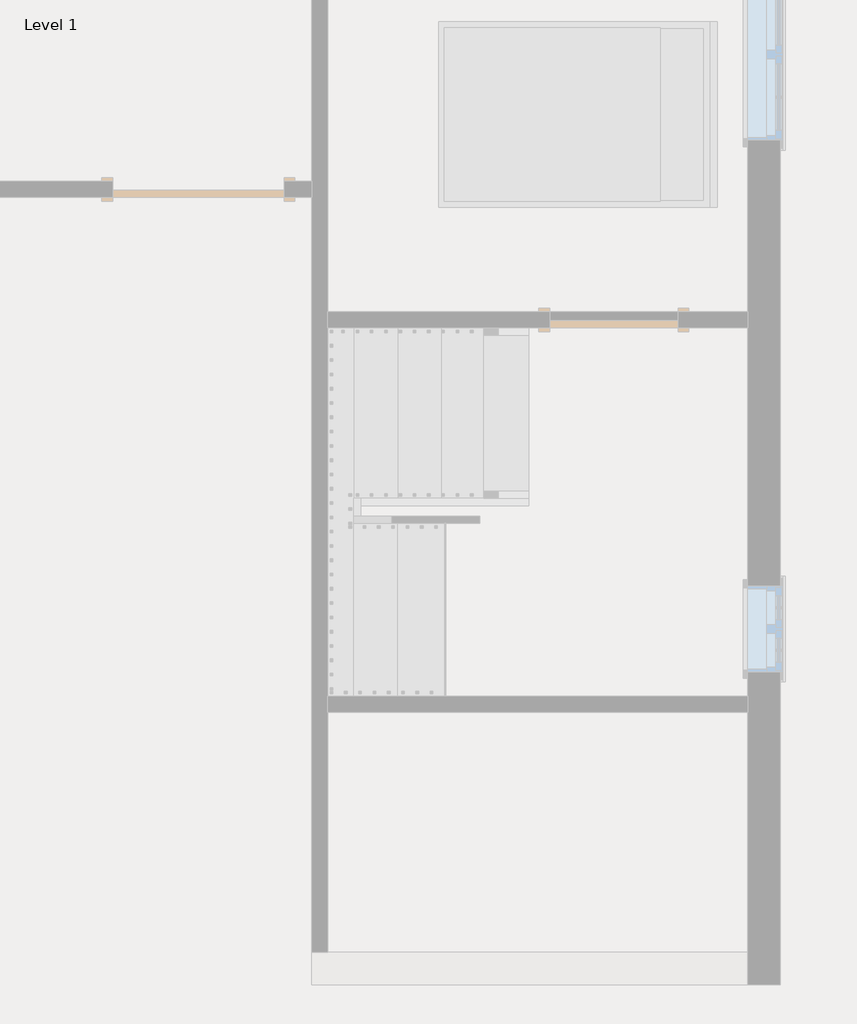
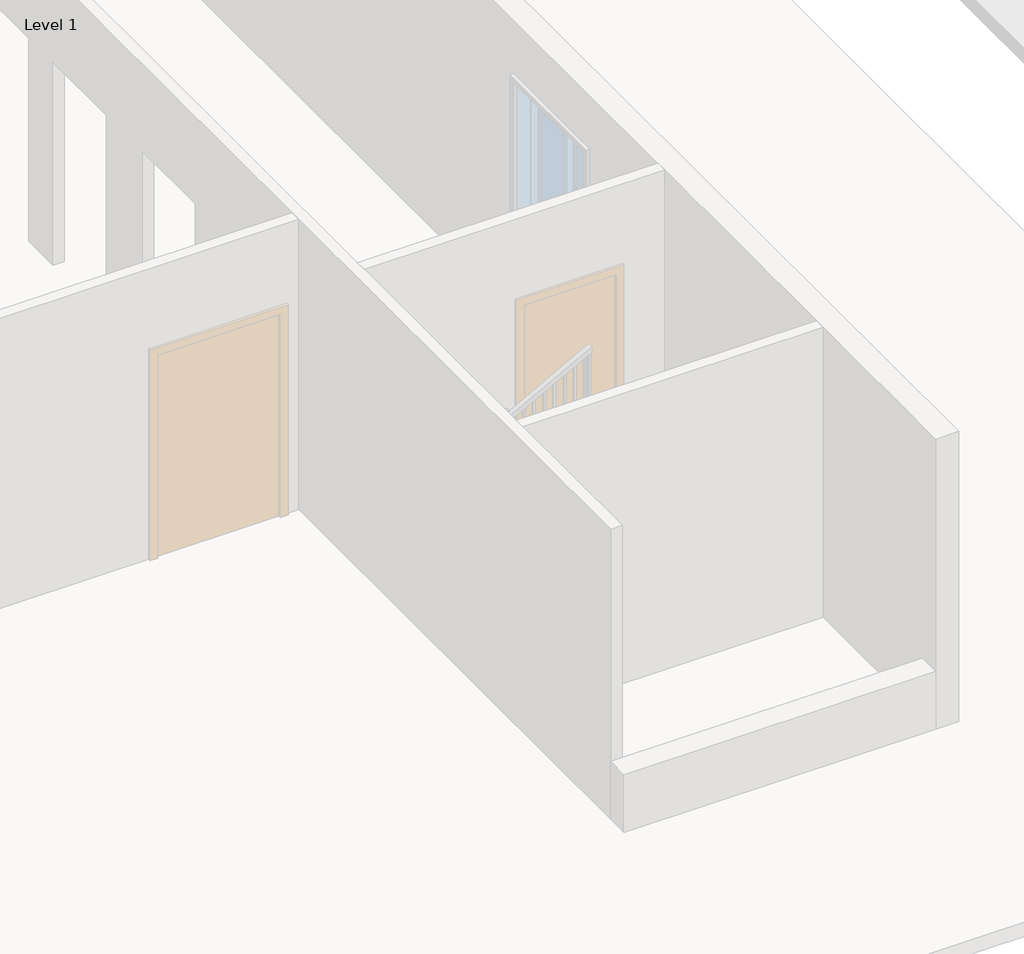
# One storey, part 5 of 7: 2 railings.
"""IFC4 building model written with IfcOpenShell, lengths in millimetres."""

from ifc_helpers import new_model, si_unit, frame, origin, place, context, project, spatial, polyline, outline, extrude, faceted_brep, element, save

model = new_model("IFC4")

# Units and contexts
model_context = context("Model", 3, world=origin())
ifc_project = project(units=[si_unit("LENGTHUNIT", "METRE", prefix="MILLI")], contexts=[model_context])

# Site, building, storey
site = spatial("IfcSite", under=ifc_project)
building = spatial("IfcBuilding", under=site)
storey = spatial("IfcBuildingStorey", under=building, Name="Level 1", Elevation=0.0)

# Railings
placement = place(None, origin())
element("IfcRailing", 1, ObjectType="Handrail - Rectangular", at=placement, inside=storey, context=model_context, shape_type="SolidModel", body=[
    faceted_brep([(7105.1820958, 5435.6, 1083.7333333), (7105.1820958, 5435.6, 1025.8977421), (7105.1820958, 5486.4, 1025.8977421), (7105.1820958, 5486.4, 1083.7333333), (5860.5820958, 5435.6, 1761.0666667), (5847.654197, 5435.6, 1710.2666667), (5847.654197, 5486.4, 1710.2666667), (5860.5820958, 5486.4, 1761.0666667), (5727.7, 5435.6, 1761.0666667), (5727.7, 5435.6, 1710.2666667), (5676.9, 5486.4, 1710.2666667), (5676.9, 5486.4, 1761.0666667), (5727.7, 2997.2, 1761.0666667), (5727.7, 2946.4, 1710.2666667), (5676.9, 2946.4, 1710.2666667), (5676.9, 2997.2, 1761.0666667), (5727.7, 2997.2, 1899.5526009), (5727.7, 2946.4, 1848.7526009), (5676.9, 2946.4, 1848.7526009), (5676.9, 2997.2, 1899.5526009), (5727.7, 2921.0, 1899.5526009), (5727.7, 2921.0, 1848.7526009), (5676.9, 2870.2, 1848.7526009), (5676.9, 2870.2, 1899.5526009), (5803.9, 2921.0, 1899.5526009), (5816.8278988, 2921.0, 1848.7526009), (5816.8278988, 2870.2, 1848.7526009), (5803.9, 2870.2, 1899.5526009), (7105.1820958, 2921.0, 2607.7333333), (7105.1820958, 2870.2, 2607.7333333), (7105.1820958, 2870.2, 2549.8977421), (7105.1820958, 2921.0, 2549.8977421)], [[[0, 1, 2, 3]], [[1, 0, 4, 5]], [[2, 1, 5, 6]], [[3, 2, 6, 7]], [[0, 3, 7, 4]], [[5, 4, 8, 9]], [[6, 5, 9, 10]], [[7, 6, 10, 11]], [[4, 7, 11, 8]], [[9, 8, 12, 13]], [[10, 9, 13, 14]], [[11, 10, 14, 15]], [[8, 11, 15, 12]], [[13, 12, 16, 17]], [[14, 13, 17, 18]], [[15, 14, 18, 19]], [[12, 15, 19, 16]], [[17, 16, 20, 21]], [[18, 17, 21, 22]], [[19, 18, 22, 23]], [[16, 19, 23, 20]], [[21, 20, 24, 25]], [[22, 21, 25, 26]], [[23, 22, 26, 27]], [[20, 23, 27, 24]], [[28, 29, 30, 31]], [[25, 24, 28, 31]], [[26, 25, 31, 30]], [[27, 26, 30, 29]], [[24, 27, 29, 28]]]),
    extrude(outline(polyline([(2510.4108873, 7032.625), (2500.0435403, 7013.575), (1524.0, 7013.575), (1524.0, 7032.625), (2510.4108873, 7032.625)])), frame((0.0, 2886.075, 0.0), z_axis=(0.0, 1.0, 0.0), x_axis=(0.0, 0.0, 1.0)), (0.0, 0.0, 1.0), 19.05),
    extrude(outline(polyline([(2455.1183703, 6931.025), (2444.7510233, 6911.975), (1524.0, 6911.975), (1524.0, 6931.025), (2455.1183703, 6931.025)])), frame((0.0, 2886.075, 0.0), z_axis=(0.0, 1.0, 0.0), x_axis=(0.0, 0.0, 1.0)), (0.0, 0.0, 1.0), 19.05),
    extrude(outline(polyline([(2399.8258533, 6829.425), (2389.4585063, 6810.375), (1524.0, 6810.375), (1524.0, 6829.425), (2399.8258533, 6829.425)])), frame((0.0, 2886.075, 0.0), z_axis=(0.0, 1.0, 0.0), x_axis=(0.0, 0.0, 1.0)), (0.0, 0.0, 1.0), 19.05),
    extrude(outline(polyline([(2344.5333363, 6727.825), (2334.1659893, 6708.775), (1354.6666667, 6708.775), (1354.6666667, 6727.825), (2344.5333363, 6727.825)])), frame((0.0, 2886.075, 0.0), z_axis=(0.0, 1.0, 0.0), x_axis=(0.0, 0.0, 1.0)), (0.0, 0.0, 1.0), 19.05),
    extrude(outline(polyline([(2289.2408192, 6626.225), (2278.8734723, 6607.175), (1354.6666667, 6607.175), (1354.6666667, 6626.225), (2289.2408192, 6626.225)])), frame((0.0, 2886.075, 0.0), z_axis=(0.0, 1.0, 0.0), x_axis=(0.0, 0.0, 1.0)), (0.0, 0.0, 1.0), 19.05),
    extrude(outline(polyline([(2233.9483022, 6524.625), (2223.5809553, 6505.575), (1354.6666667, 6505.575), (1354.6666667, 6524.625), (2233.9483022, 6524.625)])), frame((0.0, 2886.075, 0.0), z_axis=(0.0, 1.0, 0.0), x_axis=(0.0, 0.0, 1.0)), (0.0, 0.0, 1.0), 19.05),
    extrude(outline(polyline([(2178.6557852, 6423.025), (2168.2884383, 6403.975), (1185.3333333, 6403.975), (1185.3333333, 6423.025), (2178.6557852, 6423.025)])), frame((0.0, 2886.075, 0.0), z_axis=(0.0, 1.0, 0.0), x_axis=(0.0, 0.0, 1.0)), (0.0, 0.0, 1.0), 19.05),
    extrude(outline(polyline([(2123.3632682, 6321.425), (2112.9959213, 6302.375), (1185.3333333, 6302.375), (1185.3333333, 6321.425), (2123.3632682, 6321.425)])), frame((0.0, 2886.075, 0.0), z_axis=(0.0, 1.0, 0.0), x_axis=(0.0, 0.0, 1.0)), (0.0, 0.0, 1.0), 19.05),
    extrude(outline(polyline([(2068.0707512, 6219.825), (2057.7034043, 6200.775), (1185.3333333, 6200.775), (1185.3333333, 6219.825), (2068.0707512, 6219.825)])), frame((0.0, 2886.075, 0.0), z_axis=(0.0, 1.0, 0.0), x_axis=(0.0, 0.0, 1.0)), (0.0, 0.0, 1.0), 19.05),
    extrude(outline(polyline([(2012.7782342, 6118.225), (2002.4108873, 6099.175), (1016.0, 6099.175), (1016.0, 6118.225), (2012.7782342, 6118.225)])), frame((0.0, 2886.075, 0.0), z_axis=(0.0, 1.0, 0.0), x_axis=(0.0, 0.0, 1.0)), (0.0, 0.0, 1.0), 19.05),
    extrude(outline(polyline([(1957.4857172, 6016.625), (1947.1183703, 5997.575), (1016.0, 5997.575), (1016.0, 6016.625), (1957.4857172, 6016.625)])), frame((0.0, 2886.075, 0.0), z_axis=(0.0, 1.0, 0.0), x_axis=(0.0, 0.0, 1.0)), (0.0, 0.0, 1.0), 19.05),
    extrude(outline(polyline([(1902.1932002, 5915.025), (1891.8258533, 5895.975), (1016.0, 5895.975), (1016.0, 5915.025), (1902.1932002, 5915.025)])), frame((0.0, 2886.075, 0.0), z_axis=(0.0, 1.0, 0.0), x_axis=(0.0, 0.0, 1.0)), (0.0, 0.0, 1.0), 19.05),
    extrude(outline(polyline([(1846.9006832, 5813.425), (1836.5333363, 5794.375), (846.6666667, 5794.375), (846.6666667, 5813.425), (1846.9006832, 5813.425)])), frame((0.0, 2886.075, 0.0), z_axis=(0.0, 1.0, 0.0), x_axis=(0.0, 0.0, 1.0)), (0.0, 0.0, 1.0), 19.05),
    extrude(outline(polyline([(5692.775, 2930.525), (5711.825, 2930.525), (5711.825, 2911.475), (5692.775, 2911.475), (5692.775, 2930.525)])), frame((0.0, 0.0, 846.6666667), z_axis=(0.0, 0.0, 1.0), x_axis=(1.0, 0.0, 0.0)), (0.0, 0.0, 1.0), 1002.0859343),
    extrude(outline(polyline([(5692.775, 3032.125), (5711.825, 3032.125), (5711.825, 3013.075), (5692.775, 3013.075), (5692.775, 3032.125)])), frame((0.0, 0.0, 846.6666667), z_axis=(0.0, 0.0, 1.0), x_axis=(1.0, 0.0, 0.0)), (0.0, 0.0, 1.0), 863.6),
    extrude(outline(polyline([(5692.775, 3133.725), (5711.825, 3133.725), (5711.825, 3114.675), (5692.775, 3114.675), (5692.775, 3133.725)])), frame((0.0, 0.0, 846.6666667), z_axis=(0.0, 0.0, 1.0), x_axis=(1.0, 0.0, 0.0)), (0.0, 0.0, 1.0), 863.6),
    extrude(outline(polyline([(5692.775, 3235.325), (5711.825, 3235.325), (5711.825, 3216.275), (5692.775, 3216.275), (5692.775, 3235.325)])), frame((0.0, 0.0, 846.6666667), z_axis=(0.0, 0.0, 1.0), x_axis=(1.0, 0.0, 0.0)), (0.0, 0.0, 1.0), 863.6),
    extrude(outline(polyline([(5692.775, 3336.925), (5711.825, 3336.925), (5711.825, 3317.875), (5692.775, 3317.875), (5692.775, 3336.925)])), frame((0.0, 0.0, 846.6666667), z_axis=(0.0, 0.0, 1.0), x_axis=(1.0, 0.0, 0.0)), (0.0, 0.0, 1.0), 863.6),
    extrude(outline(polyline([(5692.775, 3438.525), (5711.825, 3438.525), (5711.825, 3419.475), (5692.775, 3419.475), (5692.775, 3438.525)])), frame((0.0, 0.0, 846.6666667), z_axis=(0.0, 0.0, 1.0), x_axis=(1.0, 0.0, 0.0)), (0.0, 0.0, 1.0), 863.6),
    extrude(outline(polyline([(5692.775, 3540.125), (5711.825, 3540.125), (5711.825, 3521.075), (5692.775, 3521.075), (5692.775, 3540.125)])), frame((0.0, 0.0, 846.6666667), z_axis=(0.0, 0.0, 1.0), x_axis=(1.0, 0.0, 0.0)), (0.0, 0.0, 1.0), 863.6),
    extrude(outline(polyline([(5692.775, 3641.725), (5711.825, 3641.725), (5711.825, 3622.675), (5692.775, 3622.675), (5692.775, 3641.725)])), frame((0.0, 0.0, 846.6666667), z_axis=(0.0, 0.0, 1.0), x_axis=(1.0, 0.0, 0.0)), (0.0, 0.0, 1.0), 863.6),
    extrude(outline(polyline([(5692.775, 3743.325), (5711.825, 3743.325), (5711.825, 3724.275), (5692.775, 3724.275), (5692.775, 3743.325)])), frame((0.0, 0.0, 846.6666667), z_axis=(0.0, 0.0, 1.0), x_axis=(1.0, 0.0, 0.0)), (0.0, 0.0, 1.0), 863.6),
    extrude(outline(polyline([(5692.775, 3844.925), (5711.825, 3844.925), (5711.825, 3825.875), (5692.775, 3825.875), (5692.775, 3844.925)])), frame((0.0, 0.0, 846.6666667), z_axis=(0.0, 0.0, 1.0), x_axis=(1.0, 0.0, 0.0)), (0.0, 0.0, 1.0), 863.6),
    extrude(outline(polyline([(5692.775, 3946.525), (5711.825, 3946.525), (5711.825, 3927.475), (5692.775, 3927.475), (5692.775, 3946.525)])), frame((0.0, 0.0, 846.6666667), z_axis=(0.0, 0.0, 1.0), x_axis=(1.0, 0.0, 0.0)), (0.0, 0.0, 1.0), 863.6),
    extrude(outline(polyline([(5692.775, 4048.125), (5711.825, 4048.125), (5711.825, 4029.075), (5692.775, 4029.075), (5692.775, 4048.125)])), frame((0.0, 0.0, 846.6666667), z_axis=(0.0, 0.0, 1.0), x_axis=(1.0, 0.0, 0.0)), (0.0, 0.0, 1.0), 863.6),
    extrude(outline(polyline([(5692.775, 4149.725), (5711.825, 4149.725), (5711.825, 4130.675), (5692.775, 4130.675), (5692.775, 4149.725)])), frame((0.0, 0.0, 846.6666667), z_axis=(0.0, 0.0, 1.0), x_axis=(1.0, 0.0, 0.0)), (0.0, 0.0, 1.0), 863.6),
    extrude(outline(polyline([(5692.775, 4251.325), (5711.825, 4251.325), (5711.825, 4232.275), (5692.775, 4232.275), (5692.775, 4251.325)])), frame((0.0, 0.0, 846.6666667), z_axis=(0.0, 0.0, 1.0), x_axis=(1.0, 0.0, 0.0)), (0.0, 0.0, 1.0), 863.6),
    extrude(outline(polyline([(5692.775, 4352.925), (5711.825, 4352.925), (5711.825, 4333.875), (5692.775, 4333.875), (5692.775, 4352.925)])), frame((0.0, 0.0, 846.6666667), z_axis=(0.0, 0.0, 1.0), x_axis=(1.0, 0.0, 0.0)), (0.0, 0.0, 1.0), 863.6),
    extrude(outline(polyline([(5692.775, 4454.525), (5711.825, 4454.525), (5711.825, 4435.475), (5692.775, 4435.475), (5692.775, 4454.525)])), frame((0.0, 0.0, 846.6666667), z_axis=(0.0, 0.0, 1.0), x_axis=(1.0, 0.0, 0.0)), (0.0, 0.0, 1.0), 863.6),
    extrude(outline(polyline([(5692.775, 4556.125), (5711.825, 4556.125), (5711.825, 4537.075), (5692.775, 4537.075), (5692.775, 4556.125)])), frame((0.0, 0.0, 846.6666667), z_axis=(0.0, 0.0, 1.0), x_axis=(1.0, 0.0, 0.0)), (0.0, 0.0, 1.0), 863.6),
    extrude(outline(polyline([(5692.775, 4657.725), (5711.825, 4657.725), (5711.825, 4638.675), (5692.775, 4638.675), (5692.775, 4657.725)])), frame((0.0, 0.0, 846.6666667), z_axis=(0.0, 0.0, 1.0), x_axis=(1.0, 0.0, 0.0)), (0.0, 0.0, 1.0), 863.6),
    extrude(outline(polyline([(5692.775, 4759.325), (5711.825, 4759.325), (5711.825, 4740.275), (5692.775, 4740.275), (5692.775, 4759.325)])), frame((0.0, 0.0, 846.6666667), z_axis=(0.0, 0.0, 1.0), x_axis=(1.0, 0.0, 0.0)), (0.0, 0.0, 1.0), 863.6),
    extrude(outline(polyline([(5692.775, 4860.925), (5711.825, 4860.925), (5711.825, 4841.875), (5692.775, 4841.875), (5692.775, 4860.925)])), frame((0.0, 0.0, 846.6666667), z_axis=(0.0, 0.0, 1.0), x_axis=(1.0, 0.0, 0.0)), (0.0, 0.0, 1.0), 863.6),
    extrude(outline(polyline([(5692.775, 4962.525), (5711.825, 4962.525), (5711.825, 4943.475), (5692.775, 4943.475), (5692.775, 4962.525)])), frame((0.0, 0.0, 846.6666667), z_axis=(0.0, 0.0, 1.0), x_axis=(1.0, 0.0, 0.0)), (0.0, 0.0, 1.0), 863.6),
    extrude(outline(polyline([(5692.775, 5064.125), (5711.825, 5064.125), (5711.825, 5045.075), (5692.775, 5045.075), (5692.775, 5064.125)])), frame((0.0, 0.0, 846.6666667), z_axis=(0.0, 0.0, 1.0), x_axis=(1.0, 0.0, 0.0)), (0.0, 0.0, 1.0), 863.6),
    extrude(outline(polyline([(5692.775, 5165.725), (5711.825, 5165.725), (5711.825, 5146.675), (5692.775, 5146.675), (5692.775, 5165.725)])), frame((0.0, 0.0, 846.6666667), z_axis=(0.0, 0.0, 1.0), x_axis=(1.0, 0.0, 0.0)), (0.0, 0.0, 1.0), 863.6),
    extrude(outline(polyline([(5692.775, 5267.325), (5711.825, 5267.325), (5711.825, 5248.275), (5692.775, 5248.275), (5692.775, 5267.325)])), frame((0.0, 0.0, 846.6666667), z_axis=(0.0, 0.0, 1.0), x_axis=(1.0, 0.0, 0.0)), (0.0, 0.0, 1.0), 863.6),
    extrude(outline(polyline([(5692.775, 5368.925), (5711.825, 5368.925), (5711.825, 5349.875), (5692.775, 5349.875), (5692.775, 5368.925)])), frame((0.0, 0.0, 846.6666667), z_axis=(0.0, 0.0, 1.0), x_axis=(1.0, 0.0, 0.0)), (0.0, 0.0, 1.0), 863.6),
    extrude(outline(polyline([(5793.9070958, 5470.525), (5793.9070958, 5451.475), (5774.8570958, 5451.475), (5774.8570958, 5470.525), (5793.9070958, 5470.525)])), frame((0.0, 0.0, 846.6666667), z_axis=(0.0, 0.0, 1.0), x_axis=(1.0, 0.0, 0.0)), (0.0, 0.0, 1.0), 863.6),
    extrude(outline(polyline([(1684.2242727, 5895.5070958), (1694.5916197, 5876.4570958), (677.3333333, 5876.4570958), (677.3333333, 5895.5070958), (1684.2242727, 5895.5070958)])), frame((0.0, 5451.475, 0.0), z_axis=(0.0, 1.0, 0.0), x_axis=(0.0, 0.0, 1.0)), (0.0, 0.0, 1.0), 19.05),
    extrude(outline(polyline([(1628.9317557, 5997.1070958), (1639.2991027, 5978.0570958), (677.3333333, 5978.0570958), (677.3333333, 5997.1070958), (1628.9317557, 5997.1070958)])), frame((0.0, 5451.475, 0.0), z_axis=(0.0, 1.0, 0.0), x_axis=(0.0, 0.0, 1.0)), (0.0, 0.0, 1.0), 19.05),
    extrude(outline(polyline([(1573.6392387, 6098.7070958), (1584.0065857, 6079.6570958), (677.3333333, 6079.6570958), (677.3333333, 6098.7070958), (1573.6392387, 6098.7070958)])), frame((0.0, 5451.475, 0.0), z_axis=(0.0, 1.0, 0.0), x_axis=(0.0, 0.0, 1.0)), (0.0, 0.0, 1.0), 19.05),
    extrude(outline(polyline([(1518.3467217, 6200.3070958), (1528.7140687, 6181.2570958), (508.0, 6181.2570958), (508.0, 6200.3070958), (1518.3467217, 6200.3070958)])), frame((0.0, 5451.475, 0.0), z_axis=(0.0, 1.0, 0.0), x_axis=(0.0, 0.0, 1.0)), (0.0, 0.0, 1.0), 19.05),
    extrude(outline(polyline([(1463.0542047, 6301.9070958), (1473.4215517, 6282.8570958), (508.0, 6282.8570958), (508.0, 6301.9070958), (1463.0542047, 6301.9070958)])), frame((0.0, 5451.475, 0.0), z_axis=(0.0, 1.0, 0.0), x_axis=(0.0, 0.0, 1.0)), (0.0, 0.0, 1.0), 19.05),
    extrude(outline(polyline([(1407.7616877, 6403.5070958), (1418.1290347, 6384.4570958), (508.0, 6384.4570958), (508.0, 6403.5070958), (1407.7616877, 6403.5070958)])), frame((0.0, 5451.475, 0.0), z_axis=(0.0, 1.0, 0.0), x_axis=(0.0, 0.0, 1.0)), (0.0, 0.0, 1.0), 19.05),
    extrude(outline(polyline([(1352.4691707, 6505.1070958), (1362.8365176, 6486.0570958), (338.6666667, 6486.0570958), (338.6666667, 6505.1070958), (1352.4691707, 6505.1070958)])), frame((0.0, 5451.475, 0.0), z_axis=(0.0, 1.0, 0.0), x_axis=(0.0, 0.0, 1.0)), (0.0, 0.0, 1.0), 19.05),
    extrude(outline(polyline([(1297.1766537, 6606.7070958), (1307.5440006, 6587.6570958), (338.6666667, 6587.6570958), (338.6666667, 6606.7070958), (1297.1766537, 6606.7070958)])), frame((0.0, 5451.475, 0.0), z_axis=(0.0, 1.0, 0.0), x_axis=(0.0, 0.0, 1.0)), (0.0, 0.0, 1.0), 19.05),
    extrude(outline(polyline([(1241.8841367, 6708.3070958), (1252.2514836, 6689.2570958), (338.6666667, 6689.2570958), (338.6666667, 6708.3070958), (1241.8841367, 6708.3070958)])), frame((0.0, 5451.475, 0.0), z_axis=(0.0, 1.0, 0.0), x_axis=(0.0, 0.0, 1.0)), (0.0, 0.0, 1.0), 19.05),
    extrude(outline(polyline([(1186.5916197, 6809.9070958), (1196.9589666, 6790.8570958), (169.3333333, 6790.8570958), (169.3333333, 6809.9070958), (1186.5916197, 6809.9070958)])), frame((0.0, 5451.475, 0.0), z_axis=(0.0, 1.0, 0.0), x_axis=(0.0, 0.0, 1.0)), (0.0, 0.0, 1.0), 19.05),
    extrude(outline(polyline([(1131.2991027, 6911.5070958), (1141.6664496, 6892.4570958), (169.3333333, 6892.4570958), (169.3333333, 6911.5070958), (1131.2991027, 6911.5070958)])), frame((0.0, 5451.475, 0.0), z_axis=(0.0, 1.0, 0.0), x_axis=(0.0, 0.0, 1.0)), (0.0, 0.0, 1.0), 19.05),
    extrude(outline(polyline([(1076.0065857, 7013.1070958), (1086.3739326, 6994.0570958), (169.3333333, 6994.0570958), (169.3333333, 7013.1070958), (1076.0065857, 7013.1070958)])), frame((0.0, 5451.475, 0.0), z_axis=(0.0, 1.0, 0.0), x_axis=(0.0, 0.0, 1.0)), (0.0, 0.0, 1.0), 19.05),
    extrude(outline(polyline([(5692.775, 2905.125), (5711.825, 2905.125), (5711.825, 2886.075), (5692.775, 2886.075), (5692.775, 2905.125)])), frame((0.0, 0.0, 846.6666667), z_axis=(0.0, 0.0, 1.0), x_axis=(1.0, 0.0, 0.0)), (0.0, 0.0, 1.0), 1002.0859343),
    extrude(outline(polyline([(5711.825, 5470.525), (5711.825, 5451.475), (5692.775, 5451.475), (5692.775, 5470.525), (5711.825, 5470.525)])), frame((0.0, 0.0, 846.6666667), z_axis=(0.0, 0.0, 1.0), x_axis=(1.0, 0.0, 0.0)), (0.0, 0.0, 1.0), 863.6),
    extrude(outline(polyline([(2549.8977421, 7105.1820958), (2539.5303952, 7086.1320958), (1524.0, 7086.1320958), (1524.0, 7105.1820958), (2549.8977421, 7105.1820958)])), frame((0.0, 2886.075, 0.0), z_axis=(0.0, 1.0, 0.0), x_axis=(0.0, 0.0, 1.0)), (0.0, 0.0, 1.0), 19.05),
    extrude(outline(polyline([(1025.8977421, 7105.1820958), (1036.2650891, 7086.1320958), (169.3333333, 7086.1320958), (169.3333333, 7105.1820958), (1025.8977421, 7105.1820958)])), frame((0.0, 5451.475, 0.0), z_axis=(0.0, 1.0, 0.0), x_axis=(0.0, 0.0, 1.0)), (0.0, 0.0, 1.0), 19.05),
])
element("IfcRailing", 2, ObjectType="Handrail - Rectangular", at=placement, inside=storey, context=model_context, shape_type="SolidModel", body=[
    faceted_brep([(7105.1820958, 4274.6882626, 1083.7333333), (7105.1820958, 4274.6882626, 1025.8977421), (7105.1820958, 4325.4882626, 1025.8977421), (7105.1820958, 4325.4882626, 1083.7333333), (5936.7820958, 4274.6882626, 1719.5972789), (5885.9820958, 4274.6882626, 1689.4079462), (5885.9820958, 4325.4882626, 1689.4079462), (5936.7820958, 4325.4882626, 1719.5972789), (5936.7820958, 4274.6882626, 1761.0666667), (5885.9820958, 4274.6882626, 1710.2666667), (5885.9820958, 4325.4882626, 1710.2666667), (5936.7820958, 4325.4882626, 1761.0666667), (5860.5820958, 4274.6882626, 1761.0666667), (5860.5820958, 4274.6882626, 1710.2666667), (5809.7820958, 4325.4882626, 1710.2666667), (5809.7820958, 4325.4882626, 1761.0666667), (5860.5820958, 4198.4882626, 1761.0666667), (5860.5820958, 4198.4882626, 1710.2666667), (5809.7820958, 4198.4882626, 1710.2666667), (5809.7820958, 4198.4882626, 1761.0666667), (5860.5820958, 4173.0882626, 1761.0666667), (5860.5820958, 4122.2882626, 1710.2666667), (5809.7820958, 4122.2882626, 1710.2666667), (5809.7820958, 4173.0882626, 1761.0666667), (5860.5820958, 4173.0882626, 1971.8693878), (5860.5820958, 4122.2882626, 1921.0693878), (5809.7820958, 4122.2882626, 1921.0693878), (5809.7820958, 4173.0882626, 1971.8693878), (5860.5820958, 4096.8882626, 1971.8693878), (5860.5820958, 4096.8882626, 1921.0693878), (5809.7820958, 4046.0882626, 1921.0693878), (5809.7820958, 4046.0882626, 1971.8693878), (5936.7820958, 4096.8882626, 1971.8693878), (5949.7099946, 4096.8882626, 1921.0693878), (5949.7099946, 4046.0882626, 1921.0693878), (5936.7820958, 4046.0882626, 1971.8693878), (7105.1820958, 4096.8882626, 2607.7333333), (7105.1820958, 4046.0882626, 2607.7333333), (7105.1820958, 4046.0882626, 2549.8977421), (7105.1820958, 4096.8882626, 2549.8977421)], [[[0, 1, 2, 3]], [[1, 0, 4, 5]], [[2, 1, 5, 6]], [[3, 2, 6, 7]], [[0, 3, 7, 4]], [[5, 4, 8, 9]], [[6, 5, 9, 10]], [[7, 6, 10, 11]], [[4, 7, 11, 8]], [[9, 8, 12, 13]], [[10, 9, 13, 14]], [[11, 10, 14, 15]], [[8, 11, 15, 12]], [[13, 12, 16, 17]], [[14, 13, 17, 18]], [[15, 14, 18, 19]], [[12, 15, 19, 16]], [[17, 16, 20, 21]], [[18, 17, 21, 22]], [[19, 18, 22, 23]], [[16, 19, 23, 20]], [[21, 20, 24, 25]], [[22, 21, 25, 26]], [[23, 22, 26, 27]], [[20, 23, 27, 24]], [[25, 24, 28, 29]], [[26, 25, 29, 30]], [[27, 26, 30, 31]], [[24, 27, 31, 28]], [[29, 28, 32, 33]], [[30, 29, 33, 34]], [[31, 30, 34, 35]], [[28, 31, 35, 32]], [[36, 37, 38, 39]], [[33, 32, 36, 39]], [[34, 33, 39, 38]], [[35, 34, 38, 37]], [[32, 35, 37, 36]]]),
    extrude(outline(polyline([(2517.0678102, 7044.8570958), (1524.0, 7044.8570958), (1524.0, 7063.9070958), (2527.4351571, 7063.9070958), (2517.0678102, 7044.8570958)])), frame((0.0, 4061.9632626, 0.0), z_axis=(0.0, 1.0, 0.0), x_axis=(0.0, 0.0, 1.0)), (0.0, 0.0, 1.0), 19.05),
    extrude(outline(polyline([(2461.7752932, 6943.2570958), (1524.0, 6943.2570958), (1524.0, 6962.3070958), (2472.1426401, 6962.3070958), (2461.7752932, 6943.2570958)])), frame((0.0, 4061.9632626, 0.0), z_axis=(0.0, 1.0, 0.0), x_axis=(0.0, 0.0, 1.0)), (0.0, 0.0, 1.0), 19.05),
    extrude(outline(polyline([(2406.4827761, 6841.6570958), (1524.0, 6841.6570958), (1524.0, 6860.7070958), (2416.8501231, 6860.7070958), (2406.4827761, 6841.6570958)])), frame((0.0, 4061.9632626, 0.0), z_axis=(0.0, 1.0, 0.0), x_axis=(0.0, 0.0, 1.0)), (0.0, 0.0, 1.0), 19.05),
    extrude(outline(polyline([(2351.1902591, 6740.0570958), (1354.6666667, 6740.0570958), (1354.6666667, 6759.1070958), (2361.5576061, 6759.1070958), (2351.1902591, 6740.0570958)])), frame((0.0, 4061.9632626, 0.0), z_axis=(0.0, 1.0, 0.0), x_axis=(0.0, 0.0, 1.0)), (0.0, 0.0, 1.0), 19.05),
    extrude(outline(polyline([(2295.8977421, 6638.4570958), (1354.6666667, 6638.4570958), (1354.6666667, 6657.5070958), (2306.2650891, 6657.5070958), (2295.8977421, 6638.4570958)])), frame((0.0, 4061.9632626, 0.0), z_axis=(0.0, 1.0, 0.0), x_axis=(0.0, 0.0, 1.0)), (0.0, 0.0, 1.0), 19.05),
    extrude(outline(polyline([(2240.6052251, 6536.8570958), (1354.6666667, 6536.8570958), (1354.6666667, 6555.9070958), (2250.9725721, 6555.9070958), (2240.6052251, 6536.8570958)])), frame((0.0, 4061.9632626, 0.0), z_axis=(0.0, 1.0, 0.0), x_axis=(0.0, 0.0, 1.0)), (0.0, 0.0, 1.0), 19.05),
    extrude(outline(polyline([(2185.3127081, 6435.2570958), (1185.3333333, 6435.2570958), (1185.3333333, 6454.3070958), (2195.6800551, 6454.3070958), (2185.3127081, 6435.2570958)])), frame((0.0, 4061.9632626, 0.0), z_axis=(0.0, 1.0, 0.0), x_axis=(0.0, 0.0, 1.0)), (0.0, 0.0, 1.0), 19.05),
    extrude(outline(polyline([(2130.0201911, 6333.6570958), (1185.3333333, 6333.6570958), (1185.3333333, 6352.7070958), (2140.3875381, 6352.7070958), (2130.0201911, 6333.6570958)])), frame((0.0, 4061.9632626, 0.0), z_axis=(0.0, 1.0, 0.0), x_axis=(0.0, 0.0, 1.0)), (0.0, 0.0, 1.0), 19.05),
    extrude(outline(polyline([(2074.7276741, 6232.0570958), (1185.3333333, 6232.0570958), (1185.3333333, 6251.1070958), (2085.095021, 6251.1070958), (2074.7276741, 6232.0570958)])), frame((0.0, 4061.9632626, 0.0), z_axis=(0.0, 1.0, 0.0), x_axis=(0.0, 0.0, 1.0)), (0.0, 0.0, 1.0), 19.05),
    extrude(outline(polyline([(2019.4351571, 6130.4570958), (1016.0, 6130.4570958), (1016.0, 6149.5070958), (2029.802504, 6149.5070958), (2019.4351571, 6130.4570958)])), frame((0.0, 4061.9632626, 0.0), z_axis=(0.0, 1.0, 0.0), x_axis=(0.0, 0.0, 1.0)), (0.0, 0.0, 1.0), 19.05),
    extrude(outline(polyline([(1964.1426401, 6028.8570958), (1016.0, 6028.8570958), (1016.0, 6047.9070958), (1974.509987, 6047.9070958), (1964.1426401, 6028.8570958)])), frame((0.0, 4061.9632626, 0.0), z_axis=(0.0, 1.0, 0.0), x_axis=(0.0, 0.0, 1.0)), (0.0, 0.0, 1.0), 19.05),
    extrude(outline(polyline([(1908.8501231, 5927.2570958), (1016.0, 5927.2570958), (1016.0, 5946.3070958), (1919.21747, 5946.3070958), (1908.8501231, 5927.2570958)])), frame((0.0, 4061.9632626, 0.0), z_axis=(0.0, 1.0, 0.0), x_axis=(0.0, 0.0, 1.0)), (0.0, 0.0, 1.0), 19.05),
    extrude(outline(polyline([(5844.7070958, 4106.4132626), (5844.7070958, 4087.3632626), (5825.6570958, 4087.3632626), (5825.6570958, 4106.4132626), (5844.7070958, 4106.4132626)])), frame((0.0, 0.0, 846.6666667), z_axis=(0.0, 0.0, 1.0), x_axis=(1.0, 0.0, 0.0)), (0.0, 0.0, 1.0), 1074.4027211),
    extrude(outline(polyline([(5844.7070958, 4208.0132626), (5844.7070958, 4188.9632626), (5825.6570958, 4188.9632626), (5825.6570958, 4208.0132626), (5844.7070958, 4208.0132626)])), frame((0.0, 0.0, 846.6666667), z_axis=(0.0, 0.0, 1.0), x_axis=(1.0, 0.0, 0.0)), (0.0, 0.0, 1.0), 863.6),
    extrude(outline(polyline([(5895.5070958, 4290.5632626), (5876.4570958, 4290.5632626), (5876.4570958, 4309.6132626), (5895.5070958, 4309.6132626), (5895.5070958, 4290.5632626)])), frame((0.0, 0.0, 677.3333333), z_axis=(0.0, 0.0, 1.0), x_axis=(1.0, 0.0, 0.0)), (0.0, 0.0, 1.0), 1032.9333333),
    extrude(outline(polyline([(1639.2991027, 5978.0570958), (677.3333333, 5978.0570958), (677.3333333, 5997.1070958), (1628.9317557, 5997.1070958), (1639.2991027, 5978.0570958)])), frame((0.0, 4290.5632626, 0.0), z_axis=(0.0, 1.0, 0.0), x_axis=(0.0, 0.0, 1.0)), (0.0, 0.0, 1.0), 19.05),
    extrude(outline(polyline([(1584.0065857, 6079.6570958), (677.3333333, 6079.6570958), (677.3333333, 6098.7070958), (1573.6392387, 6098.7070958), (1584.0065857, 6079.6570958)])), frame((0.0, 4290.5632626, 0.0), z_axis=(0.0, 1.0, 0.0), x_axis=(0.0, 0.0, 1.0)), (0.0, 0.0, 1.0), 19.05),
    extrude(outline(polyline([(1528.7140687, 6181.2570958), (508.0, 6181.2570958), (508.0, 6200.3070958), (1518.3467217, 6200.3070958), (1528.7140687, 6181.2570958)])), frame((0.0, 4290.5632626, 0.0), z_axis=(0.0, 1.0, 0.0), x_axis=(0.0, 0.0, 1.0)), (0.0, 0.0, 1.0), 19.05),
    extrude(outline(polyline([(1473.4215517, 6282.8570958), (508.0, 6282.8570958), (508.0, 6301.9070958), (1463.0542047, 6301.9070958), (1473.4215517, 6282.8570958)])), frame((0.0, 4290.5632626, 0.0), z_axis=(0.0, 1.0, 0.0), x_axis=(0.0, 0.0, 1.0)), (0.0, 0.0, 1.0), 19.05),
    extrude(outline(polyline([(1418.1290347, 6384.4570958), (508.0, 6384.4570958), (508.0, 6403.5070958), (1407.7616877, 6403.5070958), (1418.1290347, 6384.4570958)])), frame((0.0, 4290.5632626, 0.0), z_axis=(0.0, 1.0, 0.0), x_axis=(0.0, 0.0, 1.0)), (0.0, 0.0, 1.0), 19.05),
    extrude(outline(polyline([(1362.8365176, 6486.0570958), (338.6666667, 6486.0570958), (338.6666667, 6505.1070958), (1352.4691707, 6505.1070958), (1362.8365176, 6486.0570958)])), frame((0.0, 4290.5632626, 0.0), z_axis=(0.0, 1.0, 0.0), x_axis=(0.0, 0.0, 1.0)), (0.0, 0.0, 1.0), 19.05),
    extrude(outline(polyline([(1307.5440006, 6587.6570958), (338.6666667, 6587.6570958), (338.6666667, 6606.7070958), (1297.1766537, 6606.7070958), (1307.5440006, 6587.6570958)])), frame((0.0, 4290.5632626, 0.0), z_axis=(0.0, 1.0, 0.0), x_axis=(0.0, 0.0, 1.0)), (0.0, 0.0, 1.0), 19.05),
    extrude(outline(polyline([(1252.2514836, 6689.2570958), (338.6666667, 6689.2570958), (338.6666667, 6708.3070958), (1241.8841367, 6708.3070958), (1252.2514836, 6689.2570958)])), frame((0.0, 4290.5632626, 0.0), z_axis=(0.0, 1.0, 0.0), x_axis=(0.0, 0.0, 1.0)), (0.0, 0.0, 1.0), 19.05),
    extrude(outline(polyline([(1196.9589666, 6790.8570958), (169.3333333, 6790.8570958), (169.3333333, 6809.9070958), (1186.5916197, 6809.9070958), (1196.9589666, 6790.8570958)])), frame((0.0, 4290.5632626, 0.0), z_axis=(0.0, 1.0, 0.0), x_axis=(0.0, 0.0, 1.0)), (0.0, 0.0, 1.0), 19.05),
    extrude(outline(polyline([(1141.6664496, 6892.4570958), (169.3333333, 6892.4570958), (169.3333333, 6911.5070958), (1131.2991027, 6911.5070958), (1141.6664496, 6892.4570958)])), frame((0.0, 4290.5632626, 0.0), z_axis=(0.0, 1.0, 0.0), x_axis=(0.0, 0.0, 1.0)), (0.0, 0.0, 1.0), 19.05),
    extrude(outline(polyline([(1086.3739326, 6994.0570958), (169.3333333, 6994.0570958), (169.3333333, 7013.1070958), (1076.0065857, 7013.1070958), (1086.3739326, 6994.0570958)])), frame((0.0, 4290.5632626, 0.0), z_axis=(0.0, 1.0, 0.0), x_axis=(0.0, 0.0, 1.0)), (0.0, 0.0, 1.0), 19.05),
    extrude(outline(polyline([(5844.7070958, 4081.0132626), (5844.7070958, 4061.9632626), (5825.6570958, 4061.9632626), (5825.6570958, 4081.0132626), (5844.7070958, 4081.0132626)])), frame((0.0, 0.0, 846.6666667), z_axis=(0.0, 0.0, 1.0), x_axis=(1.0, 0.0, 0.0)), (0.0, 0.0, 1.0), 1074.4027211),
    extrude(outline(polyline([(5844.7070958, 4290.5632626), (5825.6570958, 4290.5632626), (5825.6570958, 4309.6132626), (5844.7070958, 4309.6132626), (5844.7070958, 4290.5632626)])), frame((0.0, 0.0, 846.6666667), z_axis=(0.0, 0.0, 1.0), x_axis=(1.0, 0.0, 0.0)), (0.0, 0.0, 1.0), 863.6),
    extrude(outline(polyline([(2539.5303952, 7086.1320958), (1524.0, 7086.1320958), (1524.0, 7105.1820958), (2549.8977421, 7105.1820958), (2539.5303952, 7086.1320958)])), frame((0.0, 4061.9632626, 0.0), z_axis=(0.0, 1.0, 0.0), x_axis=(0.0, 0.0, 1.0)), (0.0, 0.0, 1.0), 19.05),
    extrude(outline(polyline([(1036.2650891, 7086.1320958), (169.3333333, 7086.1320958), (169.3333333, 7105.1820958), (1025.8977421, 7105.1820958), (1036.2650891, 7086.1320958)])), frame((0.0, 4290.5632626, 0.0), z_axis=(0.0, 1.0, 0.0), x_axis=(0.0, 0.0, 1.0)), (0.0, 0.0, 1.0), 19.05),
])

save(model, "model.ifc")

# Revit data of these elements
# Type "Handrail - Rectangular"
#   Assembly Code = "C2010400"
#   built-in parameter 1008612 = 0.0416667 (stored number, unit not read)
#   built-in parameter 1008611 = 0.0416667 (stored number, unit not read)
#   built-in parameter 1008609 = 0.333333 (stored number, unit not read)
#   built-in parameter 1008604 = 0.166667 (stored number, unit not read)
#   built-in parameter 1008603 = 0.166667 (stored number, unit not read)
#   Railing Height = 3' - 0"
#   built-in parameter 1008630 = 2
#   built-in parameter 1008610 = 2
#   built-in parameter 1008618 = Baluster - Square : 3/4"
# Elements 1, 2 (IfcRailing, "Handrail - Rectangular")
#   Phase Created = New Construction
